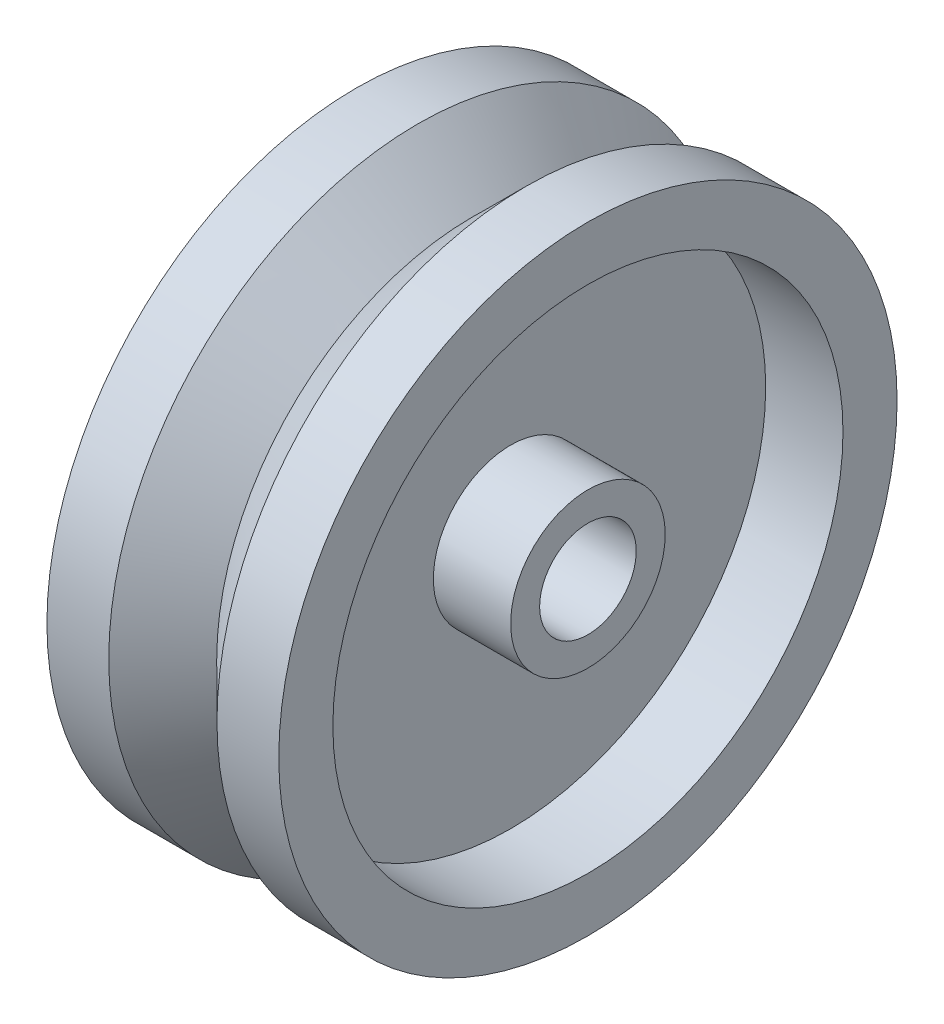
SolidWorks part; units mm, degrees
material "Plain Carbon Steel"
ref_plane "Front Plane" through (0, 0, 0) normal (0, 0, 1) x (1, 0, 0)
ref_plane "Top Plane" through (0, 0, 0) normal (0, 1, 0) x (1, 0, 0)
ref_plane "Right Plane" through (0, 0, 0) normal (1, 0, 0) x (0, 0, -1)
sketch "Wheel Profile Sketch" plane through (0, 0, 0) normal (0, 0, 1) x (1, 0, 0)
  line L0 (-7.5, -3.125) -> (7.5, -3.125)
  line L1 (0, 0) -> (41.6716, 0) construction
  line L2 (7.5, -3.125) -> (7.5, -20)
  line L3 (7.5, -20) -> (3.5, -20)
  line L4 (3.5, -20) -> (0, -16.5148)
  line L5 (0, -16.5148) -> (-3.5, -20)
  line L6 (-7.5, -3.125) -> (-7.5, -20)
  line L7 (-7.5, -20) -> (-3.5, -20)
  dimension "D1" = 15
  dimension "D2" = 3.125
  dimension "D3" = 7.5
  dimension "20" = 20
  dimension "D4" = 4
  dimension "D5" = 4
  dimension "D6" = 20
  dimension "D7" = 4.9393
revolve "Wheel Body" add sketch "Wheel Profile Sketch" angle 360 about L1
sketch "Side Recess Sketch Ø33" plane through (7.5, 0, 0) normal (1, 0, 0) x (0, 0, -1)
  circle A0 centre (0, 0) radius 5
  circle A1 centre (0, 0) radius 16.5
  dimension "D1" = 33
  dimension "10" = 10
extrude "Side Recess Ø33x5" cut sketch "Side Recess Sketch Ø33" against normal blind 5
mirror "Side Recess Mirror" about plane through (0, 0, 0) normal (1, 0, 0) of "Side Recess Ø33x5"
